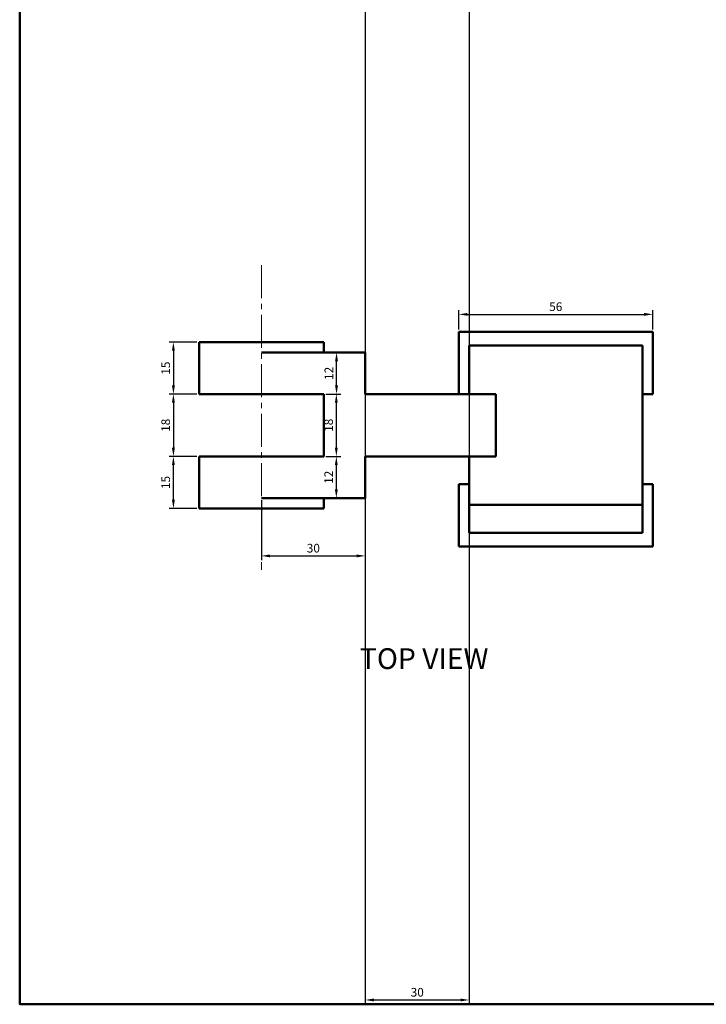
# Model space of a CAD drawing. Units: millimetres. Extents: x 1466 to 1886, y 5011 to 5605.
# Tile 1 of 4: x 1466 to 1665, y 5011 to 5295. Entities that reach past the tile are written whole.
import ezdxf

# ---------------------------------------------------------------- set-up
doc = ezdxf.new("R2010")
doc.units = ezdxf.units.MM
doc.linetypes.add('CENTER2', pattern=[28.575, 19.05, -3.175, 3.175, -3.175])
for name, color, linetype, lineweight in [('M-CNTR', 1, 'CENTER2', 18), ('M-DIMS', 2, 'Continuous', 25), ('M-OUTL', 7, 'Continuous', 50), ('M-TEXT', 7, 'Continuous', 25), ('M-TTLB', 7, 'Continuous', 50)]:
    doc.layers.add(name, color=color, linetype=linetype, lineweight=lineweight)
doc.styles.get("Standard").update_dxf_attribs({"font": 'arial.ttf'})
doc.dimstyles.new('ISO-25', dxfattribs={"dimtxt": 2.5, "dimasz": 2.5, "dimexe": 1.25, "dimexo": 0.625, "dimtad": 1, "dimtxsty": 'Standard', "dimcen": 2.5, "dimadec": 0, "dimazin": 0, "dimtfac": 1, "dimtmove": 0, "dimatfit": 3, "dimfxl": 1, "dimarcsym": 0})

# ---------------------------------------------------------------- blocks, each defined once
blk = doc.blocks.new('*D45')
at = {"layer": 'Defpoints', "color": 0, "transparency": 16777216}
for p in [(1649.06, 5209.72), (1593.06, 5204.7), (1649.06, 5204.7)]:
    blk.add_point(p, dxfattribs=at)
at = {"layer": 'M-DIMS', "color": 0, "lineweight": -2, "transparency": 16777216}
for p, q in [((1593.06, 5205.33), (1593.06, 5210.97)), ((1595.56, 5209.72), (1646.56, 5209.72)), ((1649.06, 5205.33), (1649.06, 5210.97))]:
    blk.add_line(p, q, dxfattribs=at)
at = {"layer": 'M-DIMS', "color": 0, "transparency": 16777216}
for points in [[(1595.56, 5210.14), (1595.56, 5209.3), (1593.06, 5209.72)], [(1646.56, 5210.14), (1646.56, 5209.3), (1649.06, 5209.72)]]:
    blk.add_solid(points, dxfattribs=at)
at = {"layer": 'M-DIMS', "color": 0, "transparency": 16777216, "insert": (1621.06, 5211.62), "char_height": 2.5, "attachment_point": 5}
blk.add_mtext('56', dxfattribs=at)
blk = doc.blocks.new('*D46')
at = {"layer": 'Defpoints', "color": 0, "transparency": 16777216}
for p in [(1510.65, 5168.7), (1518.06, 5168.7), (1518.06, 5153.7)]:
    blk.add_point(p, dxfattribs=at)
at = {"layer": 'M-DIMS', "color": 0, "lineweight": -2, "transparency": 16777216}
for p, q in [((1517.44, 5168.7), (1509.4, 5168.7)), ((1510.65, 5156.2), (1510.65, 5166.2)), ((1517.44, 5153.7), (1509.4, 5153.7))]:
    blk.add_line(p, q, dxfattribs=at)
at = {"layer": 'M-DIMS', "color": 0, "transparency": 16777216}
for points in [[(1510.23, 5166.2), (1511.07, 5166.2), (1510.65, 5168.7)], [(1510.23, 5156.2), (1511.07, 5156.2), (1510.65, 5153.7)]]:
    blk.add_solid(points, dxfattribs=at)
at = {"layer": 'M-DIMS', "color": 0, "transparency": 16777216, "insert": (1508.75, 5161.2), "char_height": 2.5, "attachment_point": 5, "rotation": 90}
blk.add_mtext('15', dxfattribs=at)
blk = doc.blocks.new('*D47')
at = {"layer": 'Defpoints', "color": 0, "transparency": 16777216}
for p in [(1518.06, 5186.7), (1510.65, 5168.7), (1518.06, 5168.7)]:
    blk.add_point(p, dxfattribs=at)
at = {"layer": 'M-DIMS', "color": 0, "lineweight": -2, "transparency": 16777216}
for p, q in [((1517.44, 5186.7), (1509.4, 5186.7)), ((1510.65, 5184.2), (1510.65, 5171.2)), ((1517.44, 5168.7), (1509.4, 5168.7))]:
    blk.add_line(p, q, dxfattribs=at)
at = {"layer": 'M-DIMS', "color": 0, "transparency": 16777216}
for points in [[(1510.23, 5184.2), (1511.07, 5184.2), (1510.65, 5186.7)], [(1510.23, 5171.2), (1511.07, 5171.2), (1510.65, 5168.7)]]:
    blk.add_solid(points, dxfattribs=at)
at = {"layer": 'M-DIMS', "color": 0, "transparency": 16777216, "insert": (1508.75, 5177.7), "char_height": 2.5, "attachment_point": 5, "rotation": 90}
blk.add_mtext('18', dxfattribs=at)
blk = doc.blocks.new('*D48')
at = {"layer": 'Defpoints', "color": 0, "transparency": 16777216}
for p in [(1518.06, 5201.7), (1510.65, 5186.7), (1518.06, 5186.7)]:
    blk.add_point(p, dxfattribs=at)
at = {"layer": 'M-DIMS', "color": 0, "lineweight": -2, "transparency": 16777216}
for p, q in [((1517.44, 5201.7), (1509.4, 5201.7)), ((1510.65, 5199.2), (1510.65, 5189.2)), ((1517.44, 5186.7), (1509.4, 5186.7))]:
    blk.add_line(p, q, dxfattribs=at)
at = {"layer": 'M-DIMS', "color": 0, "transparency": 16777216}
for points in [[(1510.23, 5199.2), (1511.07, 5199.2), (1510.65, 5201.7)], [(1510.23, 5189.2), (1511.07, 5189.2), (1510.65, 5186.7)]]:
    blk.add_solid(points, dxfattribs=at)
at = {"layer": 'M-DIMS', "color": 0, "transparency": 16777216, "insert": (1508.75, 5194.2), "char_height": 2.5, "attachment_point": 5, "rotation": 90}
blk.add_mtext('15', dxfattribs=at)
blk = doc.blocks.new('*D49')
at = {"layer": 'Defpoints', "color": 0, "transparency": 16777216}
for p in [(1536.06, 5156.7), (1566.06, 5156.7), (1566.06, 5140.01)]:
    blk.add_point(p, dxfattribs=at)
at = {"layer": 'M-DIMS', "color": 0, "lineweight": -2, "transparency": 16777216}
for p, q in [((1536.06, 5156.08), (1536.06, 5138.76)), ((1566.06, 5156.08), (1566.06, 5138.76)), ((1538.56, 5140.01), (1563.56, 5140.01))]:
    blk.add_line(p, q, dxfattribs=at)
at = {"layer": 'M-DIMS', "color": 0, "transparency": 16777216}
for points in [[(1538.56, 5140.42), (1538.56, 5139.59), (1536.06, 5140.01)], [(1563.56, 5140.42), (1563.56, 5139.59), (1566.06, 5140.01)]]:
    blk.add_solid(points, dxfattribs=at)
at = {"layer": 'M-DIMS', "color": 0, "transparency": 16777216, "insert": (1551.06, 5141.91), "char_height": 2.5, "attachment_point": 5}
blk.add_mtext('30', dxfattribs=at)
blk = doc.blocks.new('*D50')
at = {"layer": 'Defpoints', "color": 0, "transparency": 16777216}
for p in [(1554.06, 5186.7), (1557.7, 5186.7), (1554.06, 5168.7)]:
    blk.add_point(p, dxfattribs=at)
at = {"layer": 'M-DIMS', "color": 0, "lineweight": -2, "transparency": 16777216}
for p, q in [((1554.69, 5186.7), (1558.95, 5186.7)), ((1557.7, 5171.2), (1557.7, 5184.2)), ((1554.69, 5168.7), (1558.95, 5168.7))]:
    blk.add_line(p, q, dxfattribs=at)
at = {"layer": 'M-DIMS', "color": 0, "transparency": 16777216}
for points in [[(1557.28, 5184.2), (1558.11, 5184.2), (1557.7, 5186.7)], [(1557.28, 5171.2), (1558.11, 5171.2), (1557.7, 5168.7)]]:
    blk.add_solid(points, dxfattribs=at)
at = {"layer": 'M-DIMS', "color": 0, "transparency": 16777216, "insert": (1555.79, 5177.7), "char_height": 2.5, "attachment_point": 5, "rotation": 90}
blk.add_mtext('18', dxfattribs=at)
blk = doc.blocks.new('*D51')
at = {"layer": 'Defpoints', "color": 0, "transparency": 16777216}
for p in [(1554.06, 5198.7), (1557.75, 5198.7), (1554.06, 5186.7)]:
    blk.add_point(p, dxfattribs=at)
at = {"layer": 'M-DIMS', "color": 0, "lineweight": -2, "transparency": 16777216}
for p, q in [((1554.69, 5198.7), (1559, 5198.7)), ((1557.75, 5189.2), (1557.75, 5196.2)), ((1554.69, 5186.7), (1559, 5186.7))]:
    blk.add_line(p, q, dxfattribs=at)
at = {"layer": 'M-DIMS', "color": 0, "transparency": 16777216}
for points in [[(1557.33, 5196.2), (1558.17, 5196.2), (1557.75, 5198.7)], [(1557.33, 5189.2), (1558.17, 5189.2), (1557.75, 5186.7)]]:
    blk.add_solid(points, dxfattribs=at)
at = {"layer": 'M-DIMS', "color": 0, "transparency": 16777216, "insert": (1555.87, 5192.7), "char_height": 2.5, "attachment_point": 5, "rotation": 90}
blk.add_mtext('12', dxfattribs=at)
blk = doc.blocks.new('*D52')
at = {"layer": 'Defpoints', "color": 0, "transparency": 16777216}
for p in [(1554.06, 5168.7), (1557.7, 5168.7), (1554.06, 5156.7)]:
    blk.add_point(p, dxfattribs=at)
at = {"layer": 'M-DIMS', "color": 0, "lineweight": -2, "transparency": 16777216}
for p, q in [((1554.69, 5168.7), (1558.95, 5168.7)), ((1557.7, 5159.2), (1557.7, 5166.2)), ((1554.69, 5156.7), (1558.95, 5156.7))]:
    blk.add_line(p, q, dxfattribs=at)
at = {"layer": 'M-DIMS', "color": 0, "transparency": 16777216}
for points in [[(1557.28, 5166.2), (1558.11, 5166.2), (1557.7, 5168.7)], [(1557.28, 5159.2), (1558.11, 5159.2), (1557.7, 5156.7)]]:
    blk.add_solid(points, dxfattribs=at)
at = {"layer": 'M-DIMS', "color": 0, "transparency": 16777216, "insert": (1555.82, 5162.7), "char_height": 2.5, "attachment_point": 5, "rotation": 90}
blk.add_mtext('12', dxfattribs=at)
blk = doc.blocks.new('*D54')
at = {"layer": 'Defpoints', "color": 0, "transparency": 16777216}
for p in [(1566.06, 5505.72), (1596.06, 5505.72), (1596.06, 5011.83)]:
    blk.add_point(p, dxfattribs=at)
at = {"layer": 'M-DIMS', "color": 0, "lineweight": -2, "transparency": 16777216}
for p, q in [((1566.06, 5505.09), (1566.06, 5010.58)), ((1596.06, 5505.09), (1596.06, 5010.58)), ((1568.56, 5011.83), (1593.56, 5011.83))]:
    blk.add_line(p, q, dxfattribs=at)
at = {"layer": 'M-DIMS', "color": 0, "transparency": 16777216}
for points in [[(1568.56, 5012.25), (1568.56, 5011.41), (1566.06, 5011.83)], [(1593.56, 5012.25), (1593.56, 5011.41), (1596.06, 5011.83)]]:
    blk.add_solid(points, dxfattribs=at)
at = {"layer": 'M-DIMS', "color": 0, "transparency": 16777216, "insert": (1581.06, 5013.73), "char_height": 2.5, "attachment_point": 5}
blk.add_mtext('30', dxfattribs=at)

msp = doc.modelspace()

# ---------------------------------------------------------------- linework, layer by layer
at = {"layer": 'M-CNTR', "ltscale": 0.5}
msp.add_line((1536.065, 5223.92), (1536.065, 5135.963), dxfattribs=at)
at = {"layer": 'M-OUTL'}
for p, q in [((1649.065, 5204.701), (1593.065, 5204.701)), ((1593.065, 5204.701), (1593.065, 5186.701)), ((1649.065, 5204.701), (1649.065, 5186.701)), ((1518.065, 5186.701), (1518.065, 5201.701)), ((1518.065, 5201.701), (1554.065, 5201.701)), ((1554.065, 5201.701), (1554.065, 5198.701)), ((1566.065, 5198.701), (1536.065, 5198.701)), ((1566.065, 5198.701), (1566.065, 5186.701)), ((1596.065, 5200.701), (1596.065, 5186.701)), ((1646.065, 5200.701), (1596.065, 5200.701)), ((1646.065, 5146.701), (1646.065, 5200.701)), ((1536.065, 5186.701), (1518.065, 5186.701)), ((1554.065, 5186.701), (1536.065, 5186.701)), ((1554.065, 5186.701), (1554.065, 5168.701)), ((1596.065, 5186.701), (1566.065, 5186.701)), ((1593.065, 5186.701), (1596.065, 5186.701)), ((1596.065, 5186.701), (1603.715, 5186.701)), ((1603.715, 5186.701), (1603.715, 5168.701)), ((1649.065, 5186.701), (1646.065, 5186.701)), ((1536.065, 5168.701), (1518.065, 5168.701)), ((1518.065, 5168.701), (1518.065, 5153.701)), ((1536.065, 5168.701), (1554.065, 5168.701)), ((1566.065, 5168.701), (1596.065, 5168.701)), ((1566.065, 5156.701), (1566.065, 5168.701)), ((1596.065, 5168.701), (1596.065, 5146.701)), ((1596.065, 5168.701), (1603.715, 5168.701)), ((1593.065, 5142.701), (1593.065, 5160.701)), ((1593.065, 5160.701), (1596.065, 5160.701)), ((1649.065, 5160.701), (1646.065, 5160.701)), ((1649.065, 5142.701), (1649.065, 5160.701)), ((1536.065, 5156.701), (1566.065, 5156.701)), ((1554.065, 5153.701), (1554.065, 5156.701)), ((1518.065, 5153.701), (1554.065, 5153.701)), ((1646.065, 5154.701), (1596.065, 5154.701)), ((1596.065, 5146.701), (1646.065, 5146.701)), ((1593.065, 5142.701), (1649.065, 5142.701))]:
    msp.add_line(p, q, dxfattribs=at)
at = {"layer": 'M-TTLB'}
msp.add_lwpolyline([(1466.267, 5604.631), (1886.267, 5604.631), (1886.267, 5010.631), (1466.267, 5010.631)], close=True, dxfattribs=at)

# ---------------------------------------------------------------- texts
at = {"layer": 'M-TEXT', "insert": (1564.508, 5113.348), "char_height": 6, "attachment_point": 1}
msp.add_mtext_dynamic_manual_height_columns('TOP VIEW', width=42.55349, gutter_width=12.5, heights=[0], dxfattribs=at)

# ---------------------------------------------------------------- dimensions: what is measured, and where the dimension line sits
at = {"layer": 'M-DIMS'}
for base, p1, p2, override, picture, middle in [((1596.065, 5011.829), (1566.065, 5505.716), (1596.065, 5505.716), {"dimdec": 0, "dimlfac": 1, "dimrnd": 0, "dimzin": 0, "dimdsep": 46, "dimlunit": 2}, '*D54', (1581.065, 5013.732)), ((1649.065, 5209.72), (1593.065, 5204.701), (1649.065, 5204.701), {"dimclrd": 0, "dimclre": 0, "dimclrt": 0}, '*D45', (1621.065, 5211.621)), ((1566.065, 5140.007), (1536.065, 5156.701), (1566.065, 5156.701), {"dimclrd": 0, "dimclre": 0, "dimclrt": 0}, '*D49', (1551.065, 5141.909))]:
    dim = msp.add_linear_dim(base=base, p1=p1, p2=p2, dimstyle='ISO-25', override=override, dxfattribs=at)
    dim.commit()
    dim.dimension.update_dxf_attribs({"geometry": picture, "text_midpoint": middle})
for base, p1, p2, picture, middle in [((1510.649, 5186.701), (1518.065, 5201.701), (1518.065, 5186.701), '*D48', (1508.748, 5194.201)), ((1557.751, 5198.701), (1554.065, 5186.701), (1554.065, 5198.701), '*D51', (1555.87, 5192.701)), ((1510.649, 5168.701), (1518.065, 5186.701), (1518.065, 5168.701), '*D47', (1508.748, 5177.701)), ((1557.696, 5186.701), (1554.065, 5168.701), (1554.065, 5186.701), '*D50', (1555.795, 5177.701)), ((1510.649, 5168.701), (1518.065, 5153.701), (1518.065, 5168.701), '*D46', (1508.748, 5161.201)), ((1557.696, 5168.701), (1554.065, 5156.701), (1554.065, 5168.701), '*D52', (1555.816, 5162.701))]:
    dim = msp.add_linear_dim(base=base, p1=p1, p2=p2, angle=90, dimstyle='ISO-25', override={"dimclrd": 0, "dimclre": 0, "dimclrt": 0}, dxfattribs=at)
    dim.commit()
    dim.dimension.update_dxf_attribs({"geometry": picture, "text_midpoint": middle})

doc.saveas('drawing.dxf')
